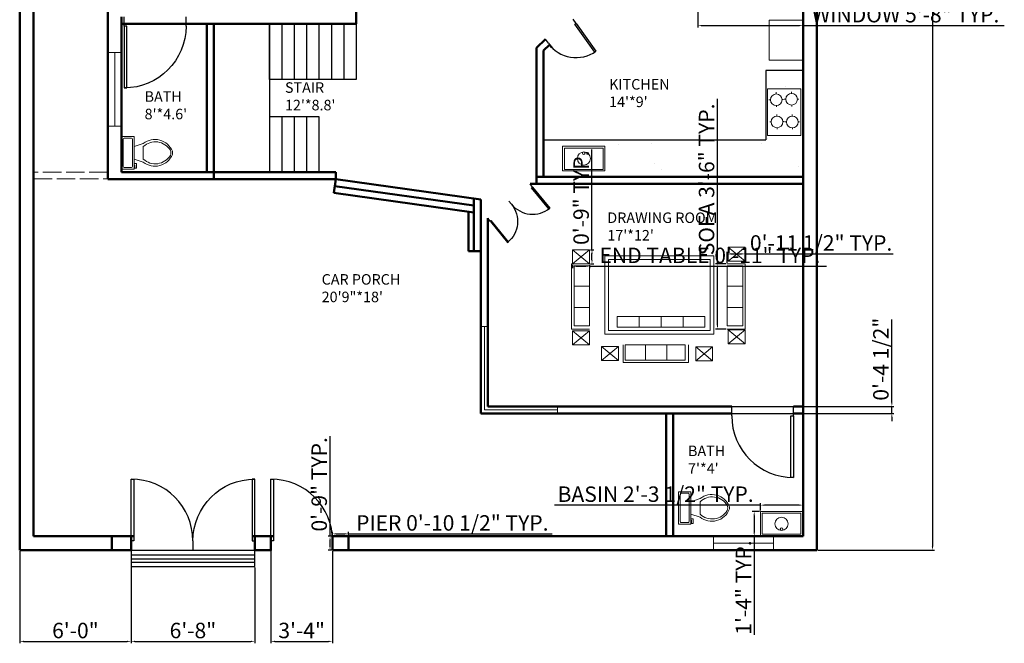
# Model space of a CAD drawing. Units: inches. Extents: x 2154 to 2791, y 2711 to 3705.
# Tile 1 of 2: x 2154 to 2791, y 2711 to 3115. Entities that reach past the tile are written whole.
import ezdxf

# ---------------------------------------------------------------- set-up
doc = ezdxf.new("R2010")
doc.units = ezdxf.units.IN
doc.linetypes.add('ACAD_ISO02W100', pattern=[15, 12, -3])
for name, color, linetype, lineweight in [('A-ANNO-DIMS', 2, 'Continuous', 18), ('A-AREA-IDEN', 104, 'Continuous', 25), ('A-COLS', 7, 'Continuous', 50), ('A-CSWK', 34, 'Continuous', 25), ('A-CSWK-PATT', 252, 'Continuous', 13), ('A-DOOR', 4, 'Continuous', 25), ('A-EQPM', 8, 'Continuous', 18), ('A-FLOR-FIXT', 9, 'Continuous', 18), ('A-FLOR-STRS', 7, 'Continuous', 25), ('A-FURN', 8, 'Continuous', 18), ('A-WALL', 7, 'Continuous', 50), ('A-WALL-OVHD', 8, 'ACAD_ISO02W100', 18), ('WINDOW', 52, 'Continuous', 18)]:
    doc.layers.add(name, color=color, linetype=linetype, lineweight=lineweight)
doc.styles.get("Standard").update_dxf_attribs({"font": 'arial.ttf'})
doc.dimstyles.new('ISO-25', dxfattribs={"dimtxt": 10, "dimasz": 2.5, "dimexe": 1.25, "dimexo": 0.625, "dimtad": 1, "dimdec": 0, "dimlunit": 4, "dimtxsty": 'Standard', "dimcen": 2.5, "dimadec": 0, "dimazin": 0, "dimtfac": 1, "dimtdec": 0, "dimtmove": 0, "dimatfit": 3, "dimfxl": 1, "dimarcsym": 0})

# ---------------------------------------------------------------- blocks, each defined once
blk = doc.blocks.new('*U2')
for p, q in [((0, 0), (0, -6)), ((40, 0), (40, -6))]:
    blk.add_line(p, q)
blk.add_lwpolyline([(0, 0), (0, 40), (1.75, 40), (1.75, 0)], close=True)
blk.add_arc((0, 0), 40, 0, 90)
blk = doc.blocks.new('*U4')
for p, q in [((9.5, -6), (9.5, -2)), ((-10, -8.5), (-8, -8.5)), ((-10, -9.5), (-10, -8.5)), ((-7, -9.5), (-10, -9.5)), ((-8, -8.5), (-8, -8)), ((-7, -8), (-7, -9.5)), ((-4, -8), (-6, -14)), ((4, -8), (6, -14)), ((4, -14), (-4, -14))]:
    blk.add_line(p, q)
blk.add_lwpolyline([(10.5, -8), (10.5, 0), (-10.5, 0), (-10.5, -8)], close=True)
for points in [[(-9.5, -2), (-9.5, -6)], [(8.5, -1), (-8.5, -1)], [(-8.5, -7), (8.5, -7)]]:
    blk.add_lwpolyline(points)
for centre, radius, start, end in [((-8.62, -1.88), 0.884, 81.8699, 188.1301), ((-8.62, -6.12), 0.884, 171.8699, 278.1301), ((8.62, -1.88), 0.884, 351.8699, 98.1301), ((8.62, -6.12), 0.884, 261.8699, 8.1301), ((3.52, -21.58), 12.17, 141.46911, 247.97143), ((4.2, -21.82), 11.33, 136.36773, 238.94682), ((-3.52, -21.58), 12.17, 292.02843, 38.53071), ((-4.2, -21.82), 11.33, 301.05301, 43.63209), ((0, -27.88), 4, 245.73182, 294.26817), ((0, -29), 4, 254.86053, 285.13947)]:
    blk.add_arc(centre, radius, start, end)
blk = doc.blocks.new('*D6')
at = {"layer": 'A-ANNO-DIMS', "color": 0, "lineweight": -2, "transparency": 16777216}
for p, q in [((2670.13, 3611.4), (2745.54, 3611.4)), ((2744.29, 3608.9), (2744.29, 2773.9)), ((2670.13, 2771.4), (2745.54, 2771.4))]:
    blk.add_line(p, q, dxfattribs=at)
at = {"layer": 'A-ANNO-DIMS', "color": 0, "lineweight": 100, "transparency": 16777216}
for points in [[(2743.87, 3608.9), (2744.7, 3608.9), (2744.29, 3611.4)], [(2743.87, 2773.9), (2744.7, 2773.9), (2744.29, 2771.4)]]:
    blk.add_solid(points, dxfattribs=at)
at = {"layer": 'Defpoints', "color": 0, "lineweight": 100, "transparency": 16777216}
for p in [(2669.51, 3611.4), (2669.51, 2771.4), (2744.29, 2771.4)]:
    blk.add_point(p, dxfattribs=at)
at = {"layer": 'A-ANNO-DIMS', "color": 0, "transparency": 16777216, "insert": (2738.56, 3191.4), "char_height": 10, "attachment_point": 5, "rotation": 90}
blk.add_mtext("70'", dxfattribs=at)
blk = doc.blocks.new('SOFA-LOUNGE-3SEAT')
for p, q in [((11.58, 42.24), (0, 42.24)), ((11.58, 0), (11.58, 42.24)), ((9.98, 27.66), (0, 27.66)), ((9.98, 13.91), (0, 13.91)), ((0, 0), (11.58, 0))]:
    blk.add_line(p, q)
blk.add_lwpolyline([(0, 2.07), (0, 40.82), (9.98, 40.82), (9.98, 2.07)], close=True)
blk = doc.blocks.new('TABLE-END-CROSSED')
for p, q in [((0, 9.07), (10.91, 0)), ((0, 0), (10.91, 9.07))]:
    blk.add_line(p, q)
blk.add_lwpolyline([(0, 9.07), (10.91, 9.07), (10.91, 0), (0, 0)], close=True)
blk = doc.blocks.new('BASIN-RECT')
for points in [[(27.46, 0), (0, 0), (0, 16.05), (27.46, 16.05)], [(1.33, 14.64), (26.38, 14.64), (26.38, 0.98), (1.33, 0.98)]]:
    blk.add_lwpolyline(points, close=True)
for centre, radius in [((13.96, 8), 4.26), ((13.84, 11.42), 0.841)]:
    blk.add_circle(centre, radius)
blk = doc.blocks.new('GATE-PIER-RECT')
blk.add_lwpolyline([(0, 0), (10.44, 0), (10.44, 9), (0, 9)], close=True)
blk = doc.blocks.new('*D16')
at = {"layer": 'A-ANNO-DIMS', "color": 0, "lineweight": -2, "transparency": 16777216}
for p, q in [((2511.37, 2956.09), (2511.37, 2953.82)), ((2513.87, 2955.07), (2519.79, 2955.07)), ((2522.29, 2956.09), (2522.29, 2953.82)), ((2522.29, 2955.07), (2675.75, 2955.07))]:
    blk.add_line(p, q, dxfattribs=at)
at = {"layer": 'A-ANNO-DIMS', "color": 0, "lineweight": 100, "transparency": 16777216}
for points in [[(2513.87, 2955.49), (2513.87, 2954.66), (2511.37, 2955.07)], [(2519.79, 2955.49), (2519.79, 2954.66), (2522.29, 2955.07)]]:
    blk.add_solid(points, dxfattribs=at)
at = {"layer": 'Defpoints', "color": 0, "lineweight": 100, "transparency": 16777216}
for p in [(2511.37, 2956.71), (2522.29, 2956.71), (2522.29, 2955.07)]:
    blk.add_point(p, dxfattribs=at)
at = {"layer": 'A-ANNO-DIMS', "color": 0, "transparency": 16777216, "insert": (2600.27, 2960.8), "char_height": 10, "attachment_point": 5}
blk.add_mtext('END TABLE 0\'-11" TYP.', dxfattribs=at)
blk = doc.blocks.new('*D17')
at = {"layer": 'A-ANNO-DIMS', "color": 0, "lineweight": -2, "transparency": 16777216}
for p, q in [((2523.92, 2965.78), (2523.92, 3030.48)), ((2522.91, 2965.78), (2525.17, 2965.78)), ((2523.92, 2959.21), (2523.92, 2963.28)), ((2522.91, 2956.71), (2525.17, 2956.71))]:
    blk.add_line(p, q, dxfattribs=at)
at = {"layer": 'A-ANNO-DIMS', "color": 0, "lineweight": 100, "transparency": 16777216}
for points in [[(2523.51, 2963.28), (2524.34, 2963.28), (2523.92, 2965.78)], [(2523.51, 2959.21), (2524.34, 2959.21), (2523.92, 2956.71)]]:
    blk.add_solid(points, dxfattribs=at)
at = {"layer": 'Defpoints', "color": 0, "lineweight": 100, "transparency": 16777216}
for p in [(2522.29, 2965.78), (2523.92, 2965.78), (2522.29, 2956.71)]:
    blk.add_point(p, dxfattribs=at)
at = {"layer": 'A-ANNO-DIMS', "color": 0, "transparency": 16777216, "insert": (2518.19, 2999.38), "char_height": 10, "attachment_point": 5, "rotation": 90}
blk.add_mtext('0\'-9" TYP.', dxfattribs=at)
blk = doc.blocks.new('*D22')
at = {"layer": 'A-ANNO-DIMS', "color": 0, "lineweight": -2, "transparency": 16777216}
for p, q in [((2605.17, 2956.71), (2605.17, 3063.28)), ((2610.88, 2956.71), (2603.92, 2956.71)), ((2605.17, 2916.97), (2605.17, 2954.21)), ((2610.88, 2914.47), (2603.92, 2914.47))]:
    blk.add_line(p, q, dxfattribs=at)
at = {"layer": 'A-ANNO-DIMS', "color": 0, "lineweight": 100, "transparency": 16777216}
for points in [[(2604.75, 2954.21), (2605.58, 2954.21), (2605.17, 2956.71)], [(2604.75, 2916.97), (2605.58, 2916.97), (2605.17, 2914.47)]]:
    blk.add_solid(points, dxfattribs=at)
at = {"layer": 'Defpoints', "color": 0, "lineweight": 100, "transparency": 16777216}
for p in [(2605.17, 2956.71), (2611.5, 2956.71), (2611.5, 2914.47)]:
    blk.add_point(p, dxfattribs=at)
at = {"layer": 'A-ANNO-DIMS', "color": 0, "transparency": 16777216, "insert": (2599.37, 3011.25), "char_height": 10, "attachment_point": 5, "rotation": 90}
blk.add_mtext('SOFA 3\'-6" TYP.', dxfattribs=at)
blk = doc.blocks.new('*D23')
at = {"layer": 'A-ANNO-DIMS', "color": 0, "lineweight": -2, "transparency": 16777216}
for p, q in [((2611.5, 2957.34), (2611.5, 2964.3)), ((2623.08, 2957.34), (2623.08, 2964.3)), ((2614, 2963.05), (2620.58, 2963.05)), ((2623.08, 2963.05), (2718.86, 2963.05))]:
    blk.add_line(p, q, dxfattribs=at)
at = {"layer": 'A-ANNO-DIMS', "color": 0, "lineweight": 100, "transparency": 16777216}
for points in [[(2614, 2963.46), (2614, 2962.63), (2611.5, 2963.05)], [(2620.58, 2963.46), (2620.58, 2962.63), (2623.08, 2963.05)]]:
    blk.add_solid(points, dxfattribs=at)
at = {"layer": 'Defpoints', "color": 0, "lineweight": 100, "transparency": 16777216}
for p in [(2623.08, 2963.05), (2611.5, 2956.71), (2623.08, 2956.71)]:
    blk.add_point(p, dxfattribs=at)
at = {"layer": 'A-ANNO-DIMS', "color": 0, "transparency": 16777216, "insert": (2672.22, 2968.84), "char_height": 10, "attachment_point": 5}
blk.add_mtext('0\'-11 1/2" TYP.', dxfattribs=at)
blk = doc.blocks.new('*D28')
at = {"layer": 'A-ANNO-DIMS', "color": 0, "lineweight": -2, "transparency": 16777216}
for p, q in [((2633.05, 2800.56), (2499.68, 2800.56)), ((2633.05, 2797.07), (2633.05, 2801.81)), ((2658.01, 2800.56), (2635.55, 2800.56)), ((2660.51, 2797.07), (2660.51, 2801.81))]:
    blk.add_line(p, q, dxfattribs=at)
at = {"layer": 'A-ANNO-DIMS', "color": 0, "lineweight": 100, "transparency": 16777216}
for points in [[(2635.55, 2800.98), (2635.55, 2800.15), (2633.05, 2800.56)], [(2658.01, 2800.98), (2658.01, 2800.15), (2660.51, 2800.56)]]:
    blk.add_solid(points, dxfattribs=at)
at = {"layer": 'Defpoints', "color": 0, "lineweight": 100, "transparency": 16777216}
for p in [(2633.05, 2800.56), (2633.05, 2796.44), (2660.51, 2796.44)]:
    blk.add_point(p, dxfattribs=at)
at = {"layer": 'A-ANNO-DIMS', "color": 0, "transparency": 16777216, "insert": (2565.12, 2806.36), "char_height": 10, "attachment_point": 5}
blk.add_mtext('BASIN 2\'-3 1/2" TYP.', dxfattribs=at)
blk = doc.blocks.new('*D29')
at = {"layer": 'A-ANNO-DIMS', "color": 0, "lineweight": -2, "transparency": 16777216}
for p, q in [((2632.42, 2796.44), (2627.68, 2796.44)), ((2628.93, 2793.94), (2628.93, 2782.9)), ((2632.42, 2780.4), (2627.68, 2780.4)), ((2628.93, 2780.4), (2628.93, 2716.63))]:
    blk.add_line(p, q, dxfattribs=at)
at = {"layer": 'A-ANNO-DIMS', "color": 0, "lineweight": 100, "transparency": 16777216}
for points in [[(2628.51, 2793.94), (2629.35, 2793.94), (2628.93, 2796.44)], [(2628.51, 2782.9), (2629.35, 2782.9), (2628.93, 2780.4)]]:
    blk.add_solid(points, dxfattribs=at)
at = {"layer": 'Defpoints', "color": 0, "lineweight": 100, "transparency": 16777216}
for p in [(2633.05, 2796.44), (2628.93, 2780.4), (2633.05, 2780.4)]:
    blk.add_point(p, dxfattribs=at)
at = {"layer": 'A-ANNO-DIMS', "color": 0, "transparency": 16777216, "insert": (2623.28, 2747.26), "char_height": 10, "attachment_point": 5, "rotation": 90}
blk.add_mtext('1\'-4" TYP.', dxfattribs=at)
blk = doc.blocks.new('*D30')
at = {"layer": 'A-ANNO-DIMS', "color": 0, "lineweight": -2, "transparency": 16777216}
for p, q in [((2592.51, 3120.27), (2592.51, 3109.45)), ((2660.51, 3120.27), (2660.51, 3109.45)), ((2595.01, 3110.7), (2658.01, 3110.7)), ((2660.51, 3110.7), (2790.8, 3110.7))]:
    blk.add_line(p, q, dxfattribs=at)
at = {"layer": 'A-ANNO-DIMS', "color": 0, "lineweight": 100, "transparency": 16777216}
for points in [[(2595.01, 3111.11), (2595.01, 3110.28), (2592.51, 3110.7)], [(2658.01, 3111.11), (2658.01, 3110.28), (2660.51, 3110.7)]]:
    blk.add_solid(points, dxfattribs=at)
at = {"layer": 'Defpoints', "color": 0, "lineweight": 100, "transparency": 16777216}
for p in [(2592.51, 3120.9), (2660.51, 3120.9), (2660.51, 3110.7)]:
    blk.add_point(p, dxfattribs=at)
at = {"layer": 'A-ANNO-DIMS', "color": 0, "transparency": 16777216, "insert": (2726.9, 3116.49), "char_height": 10, "attachment_point": 5}
blk.add_mtext('WINDOW 5\'-8" TYP.', dxfattribs=at)
blk = doc.blocks.new('*D32')
at = {"layer": 'A-ANNO-DIMS', "color": 0, "lineweight": -2, "transparency": 16777216}
for p, q in [((2355.95, 2781.02), (2355.95, 2783.21)), ((2358.45, 2781.96), (2363.89, 2781.96)), ((2366.39, 2781.02), (2366.39, 2783.21)), ((2366.39, 2781.96), (2498.15, 2781.96))]:
    blk.add_line(p, q, dxfattribs=at)
at = {"layer": 'A-ANNO-DIMS', "color": 0, "lineweight": 100, "transparency": 16777216}
for points in [[(2358.45, 2782.38), (2358.45, 2781.54), (2355.95, 2781.96)], [(2363.89, 2782.38), (2363.89, 2781.54), (2366.39, 2781.96)]]:
    blk.add_solid(points, dxfattribs=at)
at = {"layer": 'Defpoints', "color": 0, "lineweight": 100, "transparency": 16777216}
for p in [(2355.95, 2780.4), (2366.39, 2781.96), (2366.39, 2780.4)]:
    blk.add_point(p, dxfattribs=at)
at = {"layer": 'A-ANNO-DIMS', "color": 0, "transparency": 16777216, "insert": (2433.52, 2787.76), "char_height": 10, "attachment_point": 5}
blk.add_mtext('PIER 0\'-10 1/2" TYP.', dxfattribs=at)
blk = doc.blocks.new('*D33')
at = {"layer": 'A-ANNO-DIMS', "color": 0, "lineweight": -2, "transparency": 16777216}
for p, q in [((2354.39, 2780.4), (2354.39, 2845.1)), ((2355.33, 2780.4), (2353.14, 2780.4)), ((2354.39, 2773.9), (2354.39, 2777.9)), ((2355.33, 2771.4), (2353.14, 2771.4))]:
    blk.add_line(p, q, dxfattribs=at)
at = {"layer": 'A-ANNO-DIMS', "color": 0, "lineweight": 100, "transparency": 16777216}
for points in [[(2353.97, 2777.9), (2354.8, 2777.9), (2354.39, 2780.4)], [(2353.97, 2773.9), (2354.8, 2773.9), (2354.39, 2771.4)]]:
    blk.add_solid(points, dxfattribs=at)
at = {"layer": 'Defpoints', "color": 0, "lineweight": 100, "transparency": 16777216}
for p in [(2354.39, 2780.4), (2355.95, 2780.4), (2355.95, 2771.4)]:
    blk.add_point(p, dxfattribs=at)
at = {"layer": 'A-ANNO-DIMS', "color": 0, "transparency": 16777216, "insert": (2348.66, 2814), "char_height": 10, "attachment_point": 5, "rotation": 90}
blk.add_mtext('0\'-9" TYP.', dxfattribs=at)
blk = doc.blocks.new('*D34')
at = {"layer": 'A-ANNO-DIMS', "color": 0, "lineweight": -2, "transparency": 16777216}
for p, q in [((2153.51, 2770.77), (2153.51, 2711.2)), ((2225.63, 2770.77), (2225.63, 2711.2)), ((2156.01, 2712.45), (2223.13, 2712.45))]:
    blk.add_line(p, q, dxfattribs=at)
at = {"layer": 'A-ANNO-DIMS', "color": 0, "lineweight": 100, "transparency": 16777216}
for points in [[(2156.01, 2712.87), (2156.01, 2712.04), (2153.51, 2712.45)], [(2223.13, 2712.87), (2223.13, 2712.04), (2225.63, 2712.45)]]:
    blk.add_solid(points, dxfattribs=at)
at = {"layer": 'Defpoints', "color": 0, "lineweight": 100, "transparency": 16777216}
for p in [(2153.51, 2771.4), (2225.63, 2771.4), (2225.63, 2712.45)]:
    blk.add_point(p, dxfattribs=at)
at = {"layer": 'A-ANNO-DIMS', "color": 0, "transparency": 16777216, "insert": (2189.57, 2718.18), "char_height": 10, "attachment_point": 5}
blk.add_mtext('6\'-0"', dxfattribs=at)
blk = doc.blocks.new('*D35')
at = {"layer": 'A-ANNO-DIMS', "color": 0, "lineweight": -2, "transparency": 16777216}
for p, q in [((2225.63, 2760.33), (2225.63, 2711.2)), ((2305.63, 2760.33), (2305.63, 2711.2)), ((2228.13, 2712.45), (2303.13, 2712.45))]:
    blk.add_line(p, q, dxfattribs=at)
at = {"layer": 'A-ANNO-DIMS', "color": 0, "lineweight": 100, "transparency": 16777216}
for points in [[(2228.13, 2712.87), (2228.13, 2712.04), (2225.63, 2712.45)], [(2303.13, 2712.87), (2303.13, 2712.04), (2305.63, 2712.45)]]:
    blk.add_solid(points, dxfattribs=at)
at = {"layer": 'Defpoints', "color": 0, "lineweight": 100, "transparency": 16777216}
for p in [(2225.63, 2760.95), (2305.63, 2760.95), (2305.63, 2712.45)]:
    blk.add_point(p, dxfattribs=at)
at = {"layer": 'A-ANNO-DIMS', "color": 0, "transparency": 16777216, "insert": (2265.63, 2718.18), "char_height": 10, "attachment_point": 5}
blk.add_mtext('6\'-8"', dxfattribs=at)
blk = doc.blocks.new('*D36')
at = {"layer": 'A-ANNO-DIMS', "color": 0, "lineweight": -2, "transparency": 16777216}
for p, q in [((2316.07, 2770.77), (2316.07, 2711.2)), ((2355.95, 2770.77), (2355.95, 2711.2)), ((2318.57, 2712.45), (2353.45, 2712.45))]:
    blk.add_line(p, q, dxfattribs=at)
at = {"layer": 'A-ANNO-DIMS', "color": 0, "lineweight": 100, "transparency": 16777216}
for points in [[(2318.57, 2712.87), (2318.57, 2712.04), (2316.07, 2712.45)], [(2353.45, 2712.87), (2353.45, 2712.04), (2355.95, 2712.45)]]:
    blk.add_solid(points, dxfattribs=at)
at = {"layer": 'Defpoints', "color": 0, "lineweight": 100, "transparency": 16777216}
for p in [(2316.07, 2771.4), (2355.95, 2771.4), (2355.95, 2712.45)]:
    blk.add_point(p, dxfattribs=at)
at = {"layer": 'A-ANNO-DIMS', "color": 0, "transparency": 16777216, "insert": (2336.01, 2718.19), "char_height": 10, "attachment_point": 5}
blk.add_mtext('3\'-4"', dxfattribs=at)
blk = doc.blocks.new('*D39')
at = {"layer": 'A-ANNO-DIMS', "color": 0, "lineweight": -2, "transparency": 16777216}
for p, q in [((2718.01, 2866.9), (2718.01, 2920.53)), ((2457.13, 2864.4), (2719.26, 2864.4)), ((2718.01, 2859.9), (2718.01, 2864.4)), ((2452.63, 2859.9), (2719.26, 2859.9)), ((2718.01, 2857.4), (2718.01, 2854.9))]:
    blk.add_line(p, q, dxfattribs=at)
at = {"layer": 'A-ANNO-DIMS', "color": 0, "lineweight": 100, "transparency": 16777216}
for points in [[(2717.59, 2866.9), (2718.43, 2866.9), (2718.01, 2864.4)], [(2717.59, 2857.4), (2718.43, 2857.4), (2718.01, 2859.9)]]:
    blk.add_solid(points, dxfattribs=at)
at = {"layer": 'Defpoints', "color": 0, "lineweight": 100, "transparency": 16777216}
for p in [(2456.51, 2864.4), (2718.01, 2864.4), (2452.01, 2859.9)]:
    blk.add_point(p, dxfattribs=at)
at = {"layer": 'A-ANNO-DIMS', "color": 0, "transparency": 16777216, "insert": (2712.21, 2894.96), "char_height": 10, "attachment_point": 5, "rotation": 90}
blk.add_mtext('0\'-4 1/2"', dxfattribs=at)

msp = doc.modelspace()

# ---------------------------------------------------------------- hatches: boundary and pattern name
at = {"layer": 'A-CSWK-PATT'}
h = msp.add_hatch(dxfattribs=at)
h.set_pattern_fill('AR-SAND', color=256, scale=0.9)
h.paths.add_polyline_path([(2660.51, 3081.68), (2636.51, 3081.68), (2636.51, 3036.9), (2492.51, 3036.9), (2492.51, 3012.9), (2533.61, 3012.9), (2660.51, 3012.9)])
h.paths.add_polyline_path([(2637.47, 3039.62), (2637.47, 3069.74), (2659.03, 3069.74), (2659.03, 3039.62)], flags=16)
h.paths.add_polyline_path([(2647.44, 3048.42, -1), (2639.91, 3048.42, -1)], flags=0)
h.paths.add_polyline_path([(2639.46, 3062.71, -1), (2646.99, 3062.71, -1)], flags=0)
h.paths.add_polyline_path([(2657.35, 3048.35, -1), (2649.81, 3048.35, -1)], flags=0)
h.paths.add_polyline_path([(2532.21, 3016.74), (2504.75, 3016.74), (2504.75, 3032.79), (2532.21, 3032.79)], flags=16)
h.paths.add_polyline_path([(2656.91, 3063.07, -1), (2649.38, 3063.07, -1)], flags=0)
h.paths.add_polyline_path([(2531.12, 3017.72), (2506.07, 3017.72), (2506.07, 3031.38), (2531.12, 3031.38)], flags=0)
h.paths.add_polyline_path([(2519.43, 3028.16, -1), (2517.75, 3028.16, -0.394554), (2518.53, 3029, 0.402411), (2514.44, 3024.74, 1), (2522.97, 3024.74, 0.42218), (2518.59, 3029, -0.414214)], flags=0)

# ---------------------------------------------------------------- linework, layer by layer
at = {"layer": 'A-COLS'}
msp.add_lwpolyline([(2225.63, 2771.4), (2213.04, 2771.4), (2213.04, 2780.4), (2225.63, 2780.4)], close=True, dxfattribs=at)
at = {"layer": 'A-CSWK'}
for p, q in [((2660.51, 3081.68), (2636.51, 3081.68)), ((2636.51, 3081.68), (2636.51, 3036.9)), ((2492.51, 3012.9), (2492.51, 3036.9)), ((2492.51, 3036.9), (2636.51, 3036.9))]:
    msp.add_line(p, q, dxfattribs=at)
at = {"layer": 'A-EQPM'}
for p, q in [((2643.17, 3066.47), (2643.17, 3067.58)), ((2653.09, 3066.84), (2653.09, 3067.94)), ((2639.46, 3062.76), (2638.49, 3062.76)), ((2646.99, 3062.88), (2647.9, 3062.88)), ((2649.38, 3063.13), (2648.41, 3063.13)), ((2653.2, 3059.31), (2653.2, 3058.46)), ((2656.91, 3063.24), (2657.82, 3063.24)), ((2643.28, 3058.94), (2643.28, 3058.09)), ((2643.62, 3052.19), (2643.62, 3053.29)), ((2653.53, 3052.12), (2653.53, 3053.22)), ((2639.91, 3048.48), (2638.94, 3048.48)), ((2647.44, 3048.59), (2648.35, 3048.59)), ((2649.81, 3048.41), (2648.85, 3048.41)), ((2657.34, 3048.52), (2658.26, 3048.52)), ((2643.73, 3044.65), (2643.73, 3043.8)), ((2653.64, 3044.59), (2653.64, 3043.74))]:
    msp.add_line(p, q, dxfattribs=at)
for points in [[(2660.51, 3114.25), (2638.6, 3114.25), (2638.6, 3088.31), (2660.51, 3088.31)], [(2637.47, 3069.74), (2659.03, 3069.74), (2659.03, 3039.62), (2637.47, 3039.62)]]:
    msp.add_lwpolyline(points, close=True, dxfattribs=at)
for centre in [(2643.22, 3062.71), (2653.14, 3063.07), (2653.14, 3063.07), (2643.67, 3048.42), (2643.67, 3048.42), (2653.58, 3048.35), (2653.58, 3048.35)]:
    msp.add_circle(centre, 3.77, dxfattribs=at)
at = {"layer": 'A-FLOR-FIXT'}
for points in [[(2532.21, 3016.74), (2504.75, 3016.74), (2504.75, 3032.79), (2532.21, 3032.79)], [(2506.07, 3031.38), (2531.12, 3031.38), (2531.12, 3017.72), (2506.07, 3017.72)]]:
    msp.add_lwpolyline(points, close=True, dxfattribs=at)
for centre, radius in [((2518.71, 3024.74), 4.26), ((2518.59, 3028.16), 0.841)]:
    msp.add_circle(centre, radius, dxfattribs=at)
at = {"layer": 'A-FLOR-STRS'}
for p, q in [((2279.21, 3111.9), (2315.21, 3111.9)), ((2315.21, 3075.9), (2315.21, 3111.9)), ((2315.21, 3111.9), (2315.21, 3015.9)), ((2323.21, 3111.9), (2323.21, 3075.9)), ((2331.21, 3111.9), (2331.21, 3075.9)), ((2339.21, 3111.9), (2339.21, 3075.9)), ((2347.21, 3111.9), (2347.21, 3075.9)), ((2355.31, 3111.9), (2355.31, 3075.9)), ((2363.31, 3111.9), (2363.31, 3075.9)), ((2371.31, 3111.9), (2371.31, 3075.9)), ((2371.31, 3111.9), (2371.31, 3075.9)), ((2371.31, 3075.9), (2315.21, 3075.9)), ((2315.21, 3075.9), (2315.21, 3051.9)), ((2279.21, 3015.9), (2279.21, 3051.9)), ((2315.21, 3051.9), (2339.52, 3051.9)), ((2323.21, 3051.9), (2323.21, 3015.9)), ((2331.21, 3051.9), (2331.21, 3015.9)), ((2339.21, 3051.9), (2339.21, 3015.9)), ((2339.52, 3051.9), (2347.21, 3051.9)), ((2347.21, 3051.9), (2347.21, 3015.9)), ((2225.63, 2771.4), (2305.63, 2771.4)), ((2225.63, 2771.4), (2225.63, 2760.95)), ((2225.63, 2768.43), (2305.63, 2768.43)), ((2225.63, 2765.9), (2305.63, 2765.9)), ((2305.63, 2760.95), (2305.63, 2771.4)), ((2225.63, 2763.65), (2305.63, 2763.65)), ((2225.63, 2760.95), (2305.63, 2760.95))]:
    msp.add_line(p, q, dxfattribs=at)
at = {"layer": 'A-FURN'}
for p, q in [((2554.49, 2915.76), (2554.49, 2922.67)), ((2568.66, 2915.76), (2568.66, 2922.67)), ((2582.84, 2915.76), (2582.84, 2922.67)), ((2540.31, 2915.76), (2568.66, 2915.76)), ((2568.66, 2915.76), (2597.02, 2915.76))]:
    msp.add_line(p, q, dxfattribs=at)
for points in [[(2532.18, 2961.86), (2602.86, 2961.86), (2602.86, 2911.15), (2532.18, 2911.15)], [(2534.56, 2959.48), (2600.48, 2959.48), (2600.48, 2913.52), (2534.56, 2913.52)], [(2540.31, 2915.76), (2597.02, 2915.76), (2597.02, 2922.67), (2540.31, 2922.67)]]:
    msp.add_lwpolyline(points, close=True, dxfattribs=at)
at = {"layer": 'A-WALL'}
for p, q in [((2153.51, 2771.4), (2153.51, 3611.4)), ((2669.51, 3611.4), (2669.51, 2771.4)), ((2162.51, 2780.4), (2162.51, 3602.4)), ((2660.51, 3602.4), (2660.51, 2780.4)), ((2371.31, 3272.97), (2371.31, 3111.9)), ((2210.51, 3161.24), (2210.51, 3045.59)), ((2219.51, 3116.4), (2219.51, 3061.2)), ((2210.51, 3111.9), (2210.51, 3011.4)), ((2222.81, 3111.9), (2219.51, 3111.9)), ((2219.51, 3111.9), (2219.51, 3015.9)), ((2371.31, 3111.9), (2222.81, 3111.9)), ((2274.71, 3015.9), (2274.71, 3111.9)), ((2279.21, 3011.4), (2279.21, 3111.9)), ((2488.01, 3096.43), (2493.74, 3101.96)), ((2492.51, 3094.52), (2496.41, 3098.28)), ((2496.37, 3098.24), (2497.99, 3096.55)), ((2488.01, 3096.43), (2488.01, 3008.4)), ((2492.51, 3094.52), (2492.51, 3012.9)), ((2219.51, 3015.9), (2274.71, 3015.9)), ((2358.03, 3015.9), (2247.32, 3015.9)), ((2358.03, 3011.4), (2358.03, 3015.9)), ((2210.51, 3011.4), (2279.21, 3011.4)), ((2279.21, 3011.4), (2358.03, 3011.4)), ((2358.03, 3011.4), (2356.79, 3002.48)), ((2358.03, 3011.4), (2452.01, 2998.3)), ((2488.01, 3008.4), (2483.81, 3008.34)), ((2488.01, 3012.9), (2533.61, 3012.9)), ((2488.01, 3008.4), (2660.51, 3008.4)), ((2488.01, 3008.4), (2533.61, 3008.4)), ((2492.51, 3012.9), (2660.51, 3012.9)), ((2660.51, 3008.4), (2660.51, 2864.4)), ((2356.79, 3002.48), (2447.51, 2989.84)), ((2357.41, 3006.94), (2447.51, 2994.38)), ((2447.51, 2989.84), (2447.51, 2998.93)), ((2452.01, 2859.9), (2452.01, 2998.3)), ((2443.96, 2990.34), (2443.96, 2964.87)), ((2447.51, 2989.84), (2447.51, 2964.87)), ((2456.51, 2864.4), (2456.51, 2986.13)), ((2443.96, 2964.87), (2452.01, 2964.87)), ((2614.35, 2864.4), (2456.51, 2864.4)), ((2660.51, 2864.4), (2654.35, 2864.4)), ((2614.35, 2859.9), (2452.01, 2859.9)), ((2572.01, 2859.9), (2572.01, 2780.4)), ((2576.51, 2859.9), (2576.51, 2780.4)), ((2614.35, 2859.9), (2576.51, 2859.9)), ((2660.51, 2859.9), (2654.35, 2859.9)), ((2660.51, 2859.9), (2654.35, 2859.9)), ((2576.51, 2811.9), (2576.51, 2780.4)), ((2227.38, 2780.4), (2162.51, 2780.4)), ((2265.74, 2780.4), (2265.52, 2780.4)), ((2317.82, 2780.4), (2303.88, 2780.4)), ((2660.51, 2780.4), (2355.95, 2780.4)), ((2225.63, 2771.4), (2153.51, 2771.4)), ((2316.07, 2771.4), (2305.63, 2771.4)), ((2669.51, 2771.4), (2355.95, 2771.4))]:
    msp.add_line(p, q, dxfattribs=at)
at = {"layer": 'A-WALL-OVHD'}
msp.add_lwpolyline([(2210.51, 3015.9), (2162.51, 3015.9), (2162.51, 3011.52), (2210.51, 3011.52)], close=True, dxfattribs=at)
at = {"layer": 'WINDOW'}
for p, q in [((2215.01, 3093.4), (2215.01, 3045.59)), ((2454.26, 2916.05), (2454.26, 2862.15)), ((2501.64, 2862.15), (2454.26, 2862.15)), ((2602.58, 2775.9), (2641.5, 2775.9))]:
    msp.add_line(p, q, dxfattribs=at)
for points in [[(2219.51, 3093.4), (2210.51, 3093.4), (2210.51, 3045.59), (2219.51, 3045.59)], [(2602.58, 2780.4), (2641.5, 2780.4), (2641.5, 2771.4), (2602.58, 2771.4)]]:
    msp.add_lwpolyline(points, close=True, dxfattribs=at)
for points in [[(2456.51, 2864.4), (2456.51, 2916.05), (2452.01, 2916.05), (2452.01, 2859.9), (2456.51, 2859.9)], [(2456.51, 2859.9), (2501.64, 2859.9), (2501.64, 2864.4), (2456.51, 2864.4)]]:
    msp.add_lwpolyline(points, dxfattribs=at)

# ---------------------------------------------------------------- block references
at = {"layer": 'A-COLS'}
for p in [(2305.63, 2771.4), (2355.95, 2771.4)]:
    msp.add_blockref('GATE-PIER-RECT', p, dxfattribs=at)
at = {"layer": 'A-DOOR', "xscale": -1, "rotation": 180}
msp.add_blockref('*U2', (2221.16, 3110.4), dxfattribs=at)
at = {"layer": 'A-DOOR'}
for p, xscale, yscale, zscale, rotation in [((2513.65, 3112.11), 0.5524960202192207, 0.5524960202192207, 0.5524960202192207, 215.5609212162676), ((2485.48, 3006.29), 0.4399496780799891, 0.4399496780799891, 0.4399496780799891, 219.1270028426019), ((2458.17, 2984.08), -0.4399496780799891, 0.4399496780799891, 0.4399496780799891, 219.1270028426019)]:
    msp.add_blockref('*U2', p, dxfattribs=dict(at, xscale=xscale, yscale=yscale, zscale=zscale, rotation=rotation))
at = {"layer": 'A-DOOR', "rotation": 180}
msp.add_blockref('*U2', (2654.35, 2858.4), dxfattribs=at)
at = {"layer": 'A-DOOR'}
for p in [(2225.63, 2777.4), (2316.07, 2777.4)]:
    msp.add_blockref('*U2', p, dxfattribs=at)
at = {"layer": 'A-DOOR', "xscale": -1}
msp.add_blockref('*U2', (2305.63, 2777.4), dxfattribs=at)
at = {"layer": 'A-FLOR-FIXT'}
for name, p, rotation in [('*U4', (2219.51, 3028.42), 90), ('*U4', (2579.91, 2798.77), 90), ('BASIN-RECT', (2660.51, 2796.44), 180)]:
    msp.add_blockref(name, p, dxfattribs=dict(at, rotation=rotation))
at = {"layer": 'A-FURN'}
for name, p in [('TABLE-END-CROSSED', (2511.37, 2956.71)), ('TABLE-END-CROSSED', (2612.17, 2958.34)), ('SOFA-LOUNGE-3SEAT', (2611.5, 2914.47)), ('TABLE-END-CROSSED', (2511.37, 2904.32)), ('TABLE-END-CROSSED', (2612.15, 2904.79)), ('TABLE-END-CROSSED', (2530.11, 2894.19)), ('TABLE-END-CROSSED', (2591.05, 2893.85))]:
    msp.add_blockref(name, p, dxfattribs=at)
at = {"layer": 'A-FURN', "extrusion": (0, 0, -1), "zscale": -1}
msp.add_blockref('SOFA-LOUNGE-3SEAT', (-2522.29, 2914.47), dxfattribs=at)
at = {"layer": 'A-FURN', "extrusion": (0, 0, -1), "zscale": -1, "rotation": 270.0000000000002}
msp.add_blockref('SOFA-LOUNGE-3SEAT', (-2586.3, 2904.32), dxfattribs=at)

# ---------------------------------------------------------------- texts
at = {"layer": 'A-AREA-IDEN', "attachment_point": 1}
for s, insert, char_height in [("STAIR\\P12'*8.8'", (2325.21, 3074.05), 6.805), ("KITCHEN\\P14'*9'", (2535.01, 3076.15), 6.805), ("BATH\\P8'*4.6'", (2234.36, 3068.26), 6.805), ("DRAWING ROOM\\P17'*12'", (2533.87, 2989.86), 6.8045), ('CAR PORCH\\P20\'9"*18\'', (2348.96, 2949.98), 6.805), ("BATH\\P7'*4'", (2586.1, 2839.04), 6.805)]:
    msp.add_mtext_dynamic_manual_height_columns(s, width=177.5689, gutter_width=34.02, heights=[0], dxfattribs=dict(at, insert=insert, char_height=char_height))

# ---------------------------------------------------------------- dimensions: what is measured, and where the dimension line sits
at = {"layer": 'A-ANNO-DIMS'}
for base, p1, p2, override, picture, middle in [((2744.29, 2771.4), (2669.51, 3611.4), (2669.51, 2771.4), {"dimclrd": 0, "dimclre": 0, "dimclrt": 0}, '*D6', (2738.56, 3191.4)), ((2718.01, 2864.4), (2452.01, 2859.9), (2456.51, 2864.4), {"dimdec": 1, "dimlfac": 1, "dimrnd": 0, "dimzin": 1, "dimdsep": 46, "dimlunit": 4, "dimfrac": 2}, '*D39', (2712.21, 2894.96))]:
    dim = msp.add_linear_dim(base=base, p1=p1, p2=p2, angle=90, dimstyle='ISO-25', override=override, dxfattribs=at)
    dim.commit()
    dim.dimension.update_dxf_attribs({"geometry": picture, "text_midpoint": middle})
for base, p1, p2, text, picture, middle in [((2660.51, 3110.7), (2592.51, 3120.9), (2660.51, 3120.9), 'WINDOW <> TYP.', '*D30', (2726.9, 3116.49)), ((2522.29, 2955.07), (2511.37, 2956.71), (2522.29, 2956.71), 'END TABLE <> TYP.', '*D16', (2600.27, 2960.8)), ((2623.08, 2963.05), (2611.5, 2956.71), (2623.08, 2956.71), '<> TYP.', '*D23', (2672.22, 2968.84)), ((2366.39, 2781.96), (2355.95, 2780.4), (2366.39, 2780.4), 'PIER <> TYP.', '*D32', (2433.52, 2787.76))]:
    dim = msp.add_linear_dim(base=base, p1=p1, p2=p2, text=text, dimstyle='ISO-25', override={"dimdec": 1, "dimlfac": 1, "dimrnd": 0, "dimzin": 1, "dimdsep": 46, "dimlunit": 4, "dimfrac": 2}, dxfattribs=at)
    dim.commit()
    dim.dimension.update_dxf_attribs({"geometry": picture, "text_midpoint": middle})
for base, p1, p2, angle, text, picture, middle in [((2605.17, 2956.71), (2611.5, 2914.47), (2611.5, 2956.71), 90, 'SOFA <> TYP.', '*D22', (2599.37, 3011.25)), ((2523.92, 2965.78), (2522.29, 2956.71), (2522.29, 2965.78), 90, '<> TYP.', '*D17', (2518.19, 2999.38)), ((2354.39, 2780.4), (2355.95, 2771.4), (2355.95, 2780.4), 90, '<> TYP.', '*D33', (2348.66, 2814)), ((2633.05, 2800.56), (2660.51, 2796.44), (2633.05, 2796.44), 180, 'BASIN <> TYP.', '*D28', (2565.12, 2806.36)), ((2628.93, 2780.4), (2633.05, 2796.44), (2633.05, 2780.4), 270, '<> TYP.', '*D29', (2623.28, 2747.26))]:
    dim = msp.add_linear_dim(base=base, p1=p1, p2=p2, angle=angle, text=text, dimstyle='ISO-25', override={"dimdec": 1, "dimlfac": 1, "dimrnd": 0, "dimzin": 1, "dimdsep": 46, "dimlunit": 4, "dimfrac": 2}, dxfattribs=at)
    dim.commit()
    dim.dimension.update_dxf_attribs({"geometry": picture, "text_midpoint": middle})
for base, p1, p2, picture, middle in [((2225.63, 2712.45), (2153.51, 2771.4), (2225.63, 2771.4), '*D34', (2189.57, 2718.18)), ((2355.95, 2712.45), (2316.07, 2771.4), (2355.95, 2771.4), '*D36', (2336.01, 2718.19)), ((2305.63, 2712.45), (2225.63, 2760.95), (2305.63, 2760.95), '*D35', (2265.63, 2718.18))]:
    dim = msp.add_linear_dim(base=base, p1=p1, p2=p2, dimstyle='ISO-25', override={"dimdec": 1, "dimlfac": 1, "dimrnd": 0, "dimzin": 1, "dimdsep": 46, "dimlunit": 4, "dimfrac": 2}, dxfattribs=at)
    dim.commit()
    dim.dimension.update_dxf_attribs({"geometry": picture, "text_midpoint": middle})

doc.saveas('drawing.dxf')
